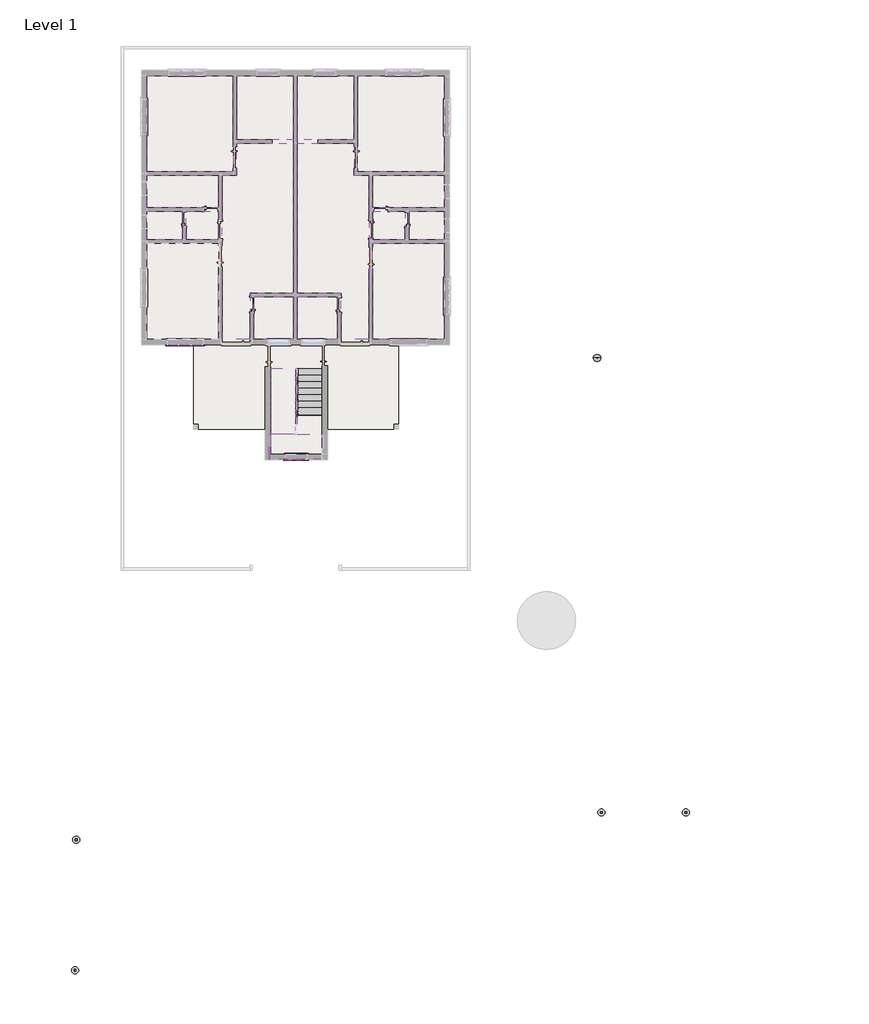
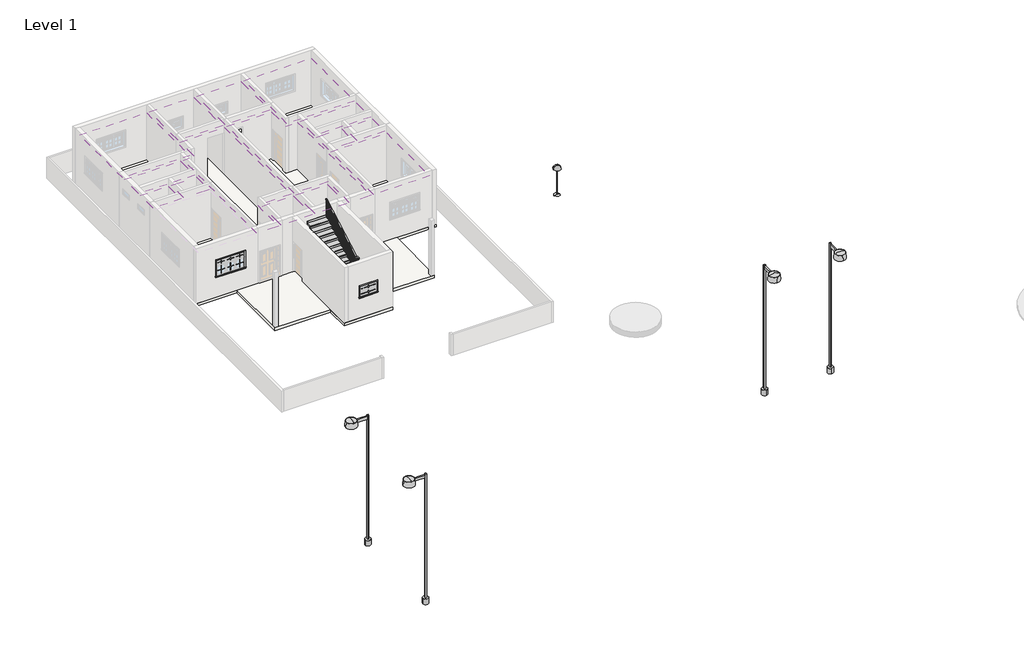
# One storey, part 3 of 4: 15 coverings, 11 proxies, 5 light fixtures, 2 slabs, 2 stair flights, 1 member, 1 railing.
"""IFC4 building model written with IfcOpenShell, lengths in millimetres."""

from ifc_helpers import new_model, si_unit, frame, origin, place, context, project, spatial, polyline, outline, extrude, faceted_brep, transform, mapped, element, save
from components import m_muntin_pattern_2x2_m_muntin_pattern_2x2_be83c6ce, m_muntin_pattern_2x2_m_muntin_pattern_2x2_d2526705, m_muntin_pattern_2x2_m_muntin_pattern_2x2_b257745b, m_muntin_pattern_2x2_m_muntin_pattern_2x2_3c44882e, m_muntin_pattern_2x2_m_muntin_pattern_2x2_c118e93d, m_trim_window_exterior_flat_with_sill_30a8f3cc, m_trim_window_exterior_flat_with_sill_78b3ef69, m_trim_window_interior_flat_picture_frame_87bc748b, m_floor_lamp_hemispheric_100w_277v_4a08ccbb, m_street_light_standard_400w_halogen_120v_204dbcbb, non_monolithic_landing_af9dc4bc, stair_flight_b7621f50, stair_flight_ccf2217f

model = new_model("IFC4")

# Units and contexts
model_context = context("Model", 3, world=origin())
ifc_project = project(units=[si_unit("LENGTHUNIT", "METRE", prefix="MILLI")], contexts=[model_context])

# Site, building, storey
site = spatial("IfcSite", under=ifc_project)
building = spatial("IfcBuilding", under=site)
storey = spatial("IfcBuildingStorey", under=building, Name="Level 1", Elevation=0.0)

# Proxies
placement = place(None, origin())
m_muntin_pattern_2x2_m_muntin_pattern_2x2_shape = m_muntin_pattern_2x2_m_muntin_pattern_2x2_be83c6ce(model_context)
element("IfcBuildingElementProxy", 1, Name="M_Muntin Pattern_2x2 : M_Muntin Pattern_2x2", ObjectType="M_Muntin Pattern_2x2 : M_Muntin Pattern_2x2", at=placement, inside=storey, context=model_context, shape_type="MappedRepresentation", body=[
    mapped(m_muntin_pattern_2x2_m_muntin_pattern_2x2_shape, transform((-11163.0966249, 7920.961641, 1289.05), x_axis=(-1.0, 0.0, 0.0), y_axis=(0.0, -1.0, 0.0), z_axis=(0.0, 0.0, 1.0))),
])
m_muntin_pattern_2x2_m_muntin_pattern_2x2_2_shape = m_muntin_pattern_2x2_m_muntin_pattern_2x2_d2526705(model_context)
element("IfcBuildingElementProxy", 2, Name="M_Muntin Pattern_2x2 : M_Muntin Pattern_2x2", ObjectType="M_Muntin Pattern_2x2 : M_Muntin Pattern_2x2", at=placement, inside=storey, context=model_context, shape_type="MappedRepresentation", body=[
    mapped(m_muntin_pattern_2x2_m_muntin_pattern_2x2_2_shape, transform((-12174.8632915, 7920.961641, 1289.05), x_axis=(1.0, 0.0, 0.0), y_axis=(0.0, 1.0, 0.0), z_axis=(0.0, 0.0, 1.0))),
])
element("IfcBuildingElementProxy", 3, Name="M_Muntin Pattern_2x2 : M_Muntin Pattern_2x2", ObjectType="M_Muntin Pattern_2x2 : M_Muntin Pattern_2x2", at=placement, inside=storey, context=model_context, shape_type="MappedRepresentation", body=[
    mapped(m_muntin_pattern_2x2_m_muntin_pattern_2x2_2_shape, transform((-11668.9799582, 7920.961641, 1289.05), x_axis=(1.0, 0.0, 0.0), y_axis=(0.0, 1.0, 0.0), z_axis=(0.0, 0.0, 1.0))),
])
m_muntin_pattern_2x2_m_muntin_pattern_2x2_3_shape = m_muntin_pattern_2x2_m_muntin_pattern_2x2_b257745b(model_context)
element("IfcBuildingElementProxy", 4, Name="M_Muntin Pattern_2x2 : M_Muntin Pattern_2x2", ObjectType="M_Muntin Pattern_2x2 : M_Muntin Pattern_2x2", at=placement, inside=storey, context=model_context, shape_type="MappedRepresentation", body=[
    mapped(m_muntin_pattern_2x2_m_muntin_pattern_2x2_3_shape, transform((-11668.9799582, 7920.961641, 1889.05), x_axis=(-1.0, 0.0, 0.0), y_axis=(0.0, -1.0, 0.0), z_axis=(0.0, 0.0, 1.0))),
])
element("IfcBuildingElementProxy", 5, Name="M_Muntin Pattern_2x2 : M_Muntin Pattern_2x2", ObjectType="M_Muntin Pattern_2x2 : M_Muntin Pattern_2x2", at=placement, inside=storey, context=model_context, shape_type="MappedRepresentation", body=[
    mapped(m_muntin_pattern_2x2_m_muntin_pattern_2x2_3_shape, transform((-12174.8632915, 7920.961641, 1889.05), x_axis=(-1.0, 0.0, 0.0), y_axis=(0.0, -1.0, 0.0), z_axis=(0.0, 0.0, 1.0))),
])
element("IfcBuildingElementProxy", 6, Name="M_Muntin Pattern_2x2 : M_Muntin Pattern_2x2", ObjectType="M_Muntin Pattern_2x2 : M_Muntin Pattern_2x2", at=placement, inside=storey, context=model_context, shape_type="MappedRepresentation", body=[
    mapped(m_muntin_pattern_2x2_m_muntin_pattern_2x2_3_shape, transform((-11163.0966249, 7920.961641, 1889.05), x_axis=(-1.0, 0.0, 0.0), y_axis=(0.0, -1.0, 0.0), z_axis=(0.0, 0.0, 1.0))),
])
m_muntin_pattern_2x2_m_muntin_pattern_2x2_4_shape = m_muntin_pattern_2x2_m_muntin_pattern_2x2_3c44882e(model_context)
element("IfcBuildingElementProxy", 7, Name="M_Muntin Pattern_2x2 : M_Muntin Pattern_2x2", ObjectType="M_Muntin Pattern_2x2 : M_Muntin Pattern_2x2", at=placement, inside=storey, context=model_context, shape_type="MappedRepresentation", body=[
    mapped(m_muntin_pattern_2x2_m_muntin_pattern_2x2_4_shape, transform((-6927.2581554, 3018.761641, 1589.05), x_axis=(-1.0, 0.0, 0.0), y_axis=(0.0, -1.0, 0.0), z_axis=(0.0, 0.0, 1.0))),
])
m_muntin_pattern_2x2_m_muntin_pattern_2x2_5_shape = m_muntin_pattern_2x2_m_muntin_pattern_2x2_c118e93d(model_context)
element("IfcBuildingElementProxy", 8, Name="M_Muntin Pattern_2x2 : M_Muntin Pattern_2x2", ObjectType="M_Muntin Pattern_2x2 : M_Muntin Pattern_2x2", at=placement, inside=storey, context=model_context, shape_type="MappedRepresentation", body=[
    mapped(m_muntin_pattern_2x2_m_muntin_pattern_2x2_5_shape, transform((-6927.2581554, 3018.761641, 1289.05), x_axis=(-1.0, 0.0, 0.0), y_axis=(0.0, -1.0, 0.0), z_axis=(0.0, 0.0, 1.0))),
])
m_trim_window_exterior_flat_with_sill_shape = m_trim_window_exterior_flat_with_sill_30a8f3cc(model_context)
element("IfcBuildingElementProxy", 9, Name="M_Trim-Window-Exterior-Flat : with Sill", ObjectType="M_Trim-Window-Exterior-Flat : with Sill", at=placement, inside=storey, context=model_context, shape_type="MappedRepresentation", body=[
    mapped(m_trim_window_exterior_flat_with_sill_shape, transform((-11668.9799582, 7911.436641, 2119.2), x_axis=(1.0, 0.0, 0.0), y_axis=(0.0, 0.0, 1.0), z_axis=(0.0, -1.0, 0.0))),
])
m_trim_window_exterior_flat_with_sill_2_shape = m_trim_window_exterior_flat_with_sill_78b3ef69(model_context)
element("IfcBuildingElementProxy", 10, Name="M_Trim-Window-Exterior-Flat : with Sill", ObjectType="M_Trim-Window-Exterior-Flat : with Sill", at=placement, inside=storey, context=model_context, shape_type="MappedRepresentation", body=[
    mapped(m_trim_window_exterior_flat_with_sill_2_shape, transform((-6927.2581554, 3009.236641, 1819.2), x_axis=(1.0, 0.0, 0.0), y_axis=(0.0, 0.0, 1.0), z_axis=(0.0, -1.0, 0.0))),
])
m_trim_window_interior_flat_picture_frame_shape = m_trim_window_interior_flat_picture_frame_87bc748b(model_context)
element("IfcBuildingElementProxy", 11, Name="M_Trim-Window-Interior-Flat : Picture Frame", ObjectType="M_Trim-Window-Interior-Flat : Picture Frame", at=placement, inside=storey, context=model_context, shape_type="MappedRepresentation", body=[
    mapped(m_trim_window_interior_flat_picture_frame_shape, transform((-6927.2581554, 3237.836641, 1819.2), x_axis=(-1.0, 0.0, 0.0), y_axis=(0.0, 0.0, 1.0), z_axis=(0.0, 1.0, 0.0))),
])

# Coverings
element("IfcCovering", 12, ObjectType="2' x 4' ACT System", at=placement, inside=storey, context=model_context, shape_type="SweptSolid", body=[
    extrude(outline(polyline([(-13313.6299582, 19417.636641), (-9630.6299582, 19417.636641), (-9630.6299582, 15302.836641), (-13313.6299582, 15302.836641), (-13313.6299582, 19417.636641)])), frame((0.0, 0.0, 2743.2), z_axis=(0.0, 0.0, 1.0), x_axis=(1.0, 0.0, 0.0)), (0.0, 0.0, 1.0), 57.15),
])
element("IfcCovering", 13, ObjectType="2' x 4' ACT System", at=placement, inside=storey, context=model_context, shape_type="SweptSolid", body=[
    extrude(outline(polyline([(-8894.0299582, 10121.236641), (-8894.0299582, 8140.036641), (-10087.8299582, 8140.036641), (-10087.8299582, 15150.436641), (-9478.2299582, 15150.436641), (-9478.2299582, 16522.036641), (-7039.8299582, 16522.036641), (-7039.8299582, 10121.236641), (-8894.0299582, 10121.236641)])), frame((0.0, 0.0, 2743.2), z_axis=(0.0, 0.0, 1.0), x_axis=(1.0, 0.0, 0.0)), (0.0, 0.0, 1.0), 57.15),
])
element("IfcCovering", 14, ObjectType="2' x 4' ACT System", at=placement, inside=storey, context=model_context, shape_type="SweptSolid", body=[
    extrude(outline(polyline([(-3814.0299582, 8140.036641), (-5007.8299582, 8140.036641), (-5007.8299582, 10121.236641), (-6887.4299582, 10121.236641), (-6887.4299582, 16522.036641), (-4449.0299582, 16522.036641), (-4449.0299582, 15150.436641), (-3814.0299582, 15150.436641), (-3814.0299582, 8140.036641)])), frame((0.0, 0.0, 2743.2), z_axis=(0.0, 0.0, 1.0), x_axis=(1.0, 0.0, 0.0)), (0.0, 0.0, 1.0), 57.15),
])
element("IfcCovering", 15, ObjectType="2' x 4' ACT System", at=placement, inside=storey, context=model_context, shape_type="SweptSolid", body=[
    extrude(outline(polyline([(-6887.4299582, 16674.436641), (-6887.4299582, 19417.636641), (-4449.0299582, 19417.636641), (-4449.0299582, 16674.436641), (-6887.4299582, 16674.436641)])), frame((0.0, 0.0, 2743.2), z_axis=(0.0, 0.0, 1.0), x_axis=(1.0, 0.0, 0.0)), (0.0, 0.0, 1.0), 57.15),
])
element("IfcCovering", 16, ObjectType="2' x 4' ACT System", at=placement, inside=storey, context=model_context, shape_type="SweptSolid", body=[
    extrude(outline(polyline([(-4296.6299582, 15302.836641), (-4296.6299582, 19417.636641), (-588.2299582, 19417.636641), (-588.2299582, 15302.836641), (-4296.6299582, 15302.836641)])), frame((0.0, 0.0, 2743.2), z_axis=(0.0, 0.0, 1.0), x_axis=(1.0, 0.0, 0.0)), (0.0, 0.0, 1.0), 57.15),
])
element("IfcCovering", 17, ObjectType="2' x 4' ACT System", at=placement, inside=storey, context=model_context, shape_type="SweptSolid", body=[
    extrude(outline(polyline([(-588.2299582, 15150.436641), (-588.2299582, 13778.836641), (-3661.6299582, 13778.836641), (-3661.6299582, 15150.436641), (-588.2299582, 15150.436641)])), frame((0.0, 0.0, 2743.2), z_axis=(0.0, 0.0, 1.0), x_axis=(1.0, 0.0, 0.0)), (0.0, 0.0, 1.0), 57.15),
])
element("IfcCovering", 18, ObjectType="2' x 4' ACT System", at=placement, inside=storey, context=model_context, shape_type="SweptSolid", body=[
    extrude(outline(polyline([(-2264.6299582, 12407.236641), (-3661.6299582, 12407.236641), (-3661.6299582, 13626.436641), (-2264.6299582, 13626.436641), (-2264.6299582, 12407.236641)])), frame((0.0, 0.0, 2743.2), z_axis=(0.0, 0.0, 1.0), x_axis=(1.0, 0.0, 0.0)), (0.0, 0.0, 1.0), 57.15),
])
element("IfcCovering", 19, ObjectType="2' x 4' ACT System", at=placement, inside=storey, context=model_context, shape_type="SweptSolid", body=[
    extrude(outline(polyline([(-2112.2299582, 13626.436641), (-588.2299582, 13626.436641), (-588.2299582, 12407.236641), (-2112.2299582, 12407.236641), (-2112.2299582, 13626.436641)])), frame((0.0, 0.0, 2743.2), z_axis=(0.0, 0.0, 1.0), x_axis=(1.0, 0.0, 0.0)), (0.0, 0.0, 1.0), 57.15),
])
element("IfcCovering", 20, ObjectType="2' x 4' ACT System", at=placement, inside=storey, context=model_context, shape_type="SweptSolid", body=[
    extrude(outline(polyline([(-588.2299582, 12254.836641), (-588.2299582, 8140.036641), (-3661.6299582, 8140.036641), (-3661.6299582, 12254.836641), (-588.2299582, 12254.836641)])), frame((0.0, 0.0, 2743.2), z_axis=(0.0, 0.0, 1.0), x_axis=(1.0, 0.0, 0.0)), (0.0, 0.0, 1.0), 57.15),
])
element("IfcCovering", 21, ObjectType="2' x 4' ACT System", at=placement, inside=storey, context=model_context, shape_type="SweptSolid", body=[
    extrude(outline(polyline([(-5160.2299582, 8140.036641), (-6887.4299582, 8140.036641), (-6887.4299582, 9968.836641), (-5160.2299582, 9968.836641), (-5160.2299582, 8140.036641)])), frame((0.0, 0.0, 2743.2), z_axis=(0.0, 0.0, 1.0), x_axis=(1.0, 0.0, 0.0)), (0.0, 0.0, 1.0), 57.15),
])
element("IfcCovering", 22, ObjectType="2' x 4' ACT System", at=placement, inside=storey, context=model_context, shape_type="SweptSolid", body=[
    extrude(outline(polyline([(-7039.8299582, 8140.036641), (-8741.6299582, 8140.036641), (-8741.6299582, 9968.836641), (-7039.8299582, 9968.836641), (-7039.8299582, 8140.036641)])), frame((0.0, 0.0, 2743.2), z_axis=(0.0, 0.0, 1.0), x_axis=(1.0, 0.0, 0.0)), (0.0, 0.0, 1.0), 57.15),
])
element("IfcCovering", 23, ObjectType="2' x 4' ACT System", at=placement, inside=storey, context=model_context, shape_type="SweptSolid", body=[
    extrude(outline(polyline([(-13313.6299582, 12407.236641), (-13313.6299582, 13626.436641), (-11776.9299582, 13626.436641), (-11776.9299582, 12407.236641), (-13313.6299582, 12407.236641)])), frame((0.0, 0.0, 2743.2), z_axis=(0.0, 0.0, 1.0), x_axis=(1.0, 0.0, 0.0)), (0.0, 0.0, 1.0), 57.15),
])
element("IfcCovering", 24, ObjectType="2' x 4' ACT System", at=placement, inside=storey, context=model_context, shape_type="SweptSolid", body=[
    extrude(outline(polyline([(-10240.2299582, 13626.436641), (-10240.2299582, 12407.236641), (-11624.5299582, 12407.236641), (-11624.5299582, 13626.436641), (-10240.2299582, 13626.436641)])), frame((0.0, 0.0, 2743.2), z_axis=(0.0, 0.0, 1.0), x_axis=(1.0, 0.0, 0.0)), (0.0, 0.0, 1.0), 57.15),
])
element("IfcCovering", 25, ObjectType="2' x 4' ACT System", at=placement, inside=storey, context=model_context, shape_type="SweptSolid", body=[
    extrude(outline(polyline([(-10240.2299582, 13778.836641), (-13313.6299582, 13778.836641), (-13313.6299582, 15150.436641), (-10240.2299582, 15150.436641), (-10240.2299582, 13778.836641)])), frame((0.0, 0.0, 2743.2), z_axis=(0.0, 0.0, 1.0), x_axis=(1.0, 0.0, 0.0)), (0.0, 0.0, 1.0), 57.15),
])
element("IfcCovering", 26, ObjectType="2' x 4' ACT System", at=placement, inside=storey, context=model_context, shape_type="SweptSolid", body=[
    extrude(outline(polyline([(-9478.2299582, 16674.436641), (-9478.2299582, 19417.636641), (-7039.8299582, 19417.636641), (-7039.8299582, 16674.436641), (-9478.2299582, 16674.436641)])), frame((0.0, 0.0, 2743.2), z_axis=(0.0, 0.0, 1.0), x_axis=(1.0, 0.0, 0.0)), (0.0, 0.0, 1.0), 57.15),
])

# Light fixtures
m_floor_lamp_hemispheric_100w_277v_shape = m_floor_lamp_hemispheric_100w_277v_4a08ccbb(model_context)
element("IfcLightFixture", 27, ObjectType="M_Floor Lamp - Hemispheric : 100W - 277V", at=placement, inside=storey, context=model_context, shape_type="MappedRepresentation", body=[
    mapped(m_floor_lamp_hemispheric_100w_277v_shape, transform((5939.5700418, 7352.636641, -141.6133158), x_axis=(1.0, 0.0, 0.0), y_axis=(0.0, 1.0, 0.0), z_axis=(0.0, 0.0, 1.0))),
])
m_street_light_standard_400w_halogen_120v_shape = m_street_light_standard_400w_halogen_120v_204dbcbb(model_context)
element("IfcLightFixture", 28, ObjectType="M_Street Light - Standard : 400W Halogen - 120V", at=placement, inside=storey, context=model_context, shape_type="MappedRepresentation", body=[
    mapped(m_street_light_standard_400w_halogen_120v_shape, transform((6127.5437539, -12075.4373856, 0.0), x_axis=(0.0, 1.0, 0.0), y_axis=(-1.0, 0.0, 0.0), z_axis=(0.0, 0.0, 1.0))),
])
element("IfcLightFixture", 29, ObjectType="M_Street Light - Standard : 400W Halogen - 120V", at=placement, inside=storey, context=model_context, shape_type="MappedRepresentation", body=[
    mapped(m_street_light_standard_400w_halogen_120v_shape, transform((9737.5760678, -12075.4373856, 0.0), x_axis=(0.0, 1.0, 0.0), y_axis=(-1.0, 0.0, 0.0), z_axis=(0.0, 0.0, 1.0))),
])
element("IfcLightFixture", 30, ObjectType="M_Street Light - Standard : 400W Halogen - 480V", at=placement, inside=storey, context=model_context, shape_type="MappedRepresentation", body=[
    mapped(m_street_light_standard_400w_halogen_120v_shape, transform((-16336.2299582, -13246.763359, -152.4), x_axis=(1.0, 0.0, 0.0), y_axis=(0.0, 1.0, 0.0), z_axis=(0.0, 0.0, 1.0))),
])
element("IfcLightFixture", 31, ObjectType="M_Street Light - Standard : 400W Halogen - 480V", at=placement, inside=storey, context=model_context, shape_type="MappedRepresentation", body=[
    mapped(m_street_light_standard_400w_halogen_120v_shape, transform((-16386.7490049, -18825.9765537, -152.4), x_axis=(1.0, 0.0, 0.0), y_axis=(0.0, 1.0, 0.0), z_axis=(0.0, 0.0, 1.0))),
])

# Member
element("IfcMember", 32, ObjectType="Stringer - 2\" Width", at=placement, inside=storey, context=model_context, shape_type="SweptSolid", body=[
    extrude(outline(polyline([(-8082.9581554, 4095.086641), (-8032.1581554, 4095.086641), (-8032.1581554, 3028.286641), (-8082.9581554, 3028.286641), (-8082.9581554, 4095.086641)])), frame((0.0, 0.0, 1524.0), z_axis=(0.0, 0.0, 1.0), x_axis=(1.0, 0.0, 0.0)), (0.0, 0.0, 1.0), 304.8),
])

# Railing
element("IfcRailing", 33, ObjectType="Handrail - Rectangular", at=placement, inside=storey, context=model_context, shape_type="SolidModel", body=[
    faceted_brep([(-6838.3581554, 6889.086641, 1073.7272727), (-6838.3581554, 6889.086641, 1015.2480499), (-6889.1581554, 6889.086641, 1015.2480499), (-6889.1581554, 6889.086641, 1073.7272727), (-6838.3581554, 4171.286641, 2623.5471074), (-6838.3581554, 4120.486641, 2594.0364797), (-6889.1581554, 4120.486641, 2594.0364797), (-6889.1581554, 4171.286641, 2623.5471074), (-6838.3581554, 4171.286641, 2667.0), (-6838.3581554, 4120.486641, 2616.2), (-6889.1581554, 4120.486641, 2616.2), (-6889.1581554, 4171.286641, 2667.0), (-6838.3581554, 4044.286641, 2667.0), (-6838.3581554, 4044.286641, 2616.2), (-6889.1581554, 4095.086641, 2616.2), (-6889.1581554, 4095.086641, 2667.0), (-6965.3581554, 4044.286641, 2667.0), (-6965.3581554, 4044.286641, 2616.2), (-6965.3581554, 4095.086641, 2616.2), (-6965.3581554, 4095.086641, 2667.0), (-6990.7581554, 4044.286641, 2667.0), (-6990.7581554, 4095.086641, 2667.0), (-6990.7581554, 4095.086641, 2616.2), (-6990.7581554, 4044.286641, 2616.2)], [[[0, 1, 2, 3]], [[1, 0, 4, 5]], [[2, 1, 5, 6]], [[3, 2, 6, 7]], [[0, 3, 7, 4]], [[5, 4, 8, 9]], [[6, 5, 9, 10]], [[7, 6, 10, 11]], [[4, 7, 11, 8]], [[9, 8, 12, 13]], [[10, 9, 13, 14]], [[11, 10, 14, 15]], [[8, 11, 15, 12]], [[13, 12, 16, 17]], [[14, 13, 17, 18]], [[15, 14, 18, 19]], [[12, 15, 19, 16]], [[20, 21, 22, 23]], [[17, 16, 20, 23]], [[18, 17, 23, 22]], [[19, 18, 22, 21]], [[16, 19, 21, 20]]]),
    faceted_brep([(-6965.3581554, 4044.286641, 2667.0), (-7016.1581554, 4044.286641, 2616.2), (-7016.1581554, 4095.086641, 2616.2), (-6965.3581554, 4095.086641, 2667.0), (-6965.3581554, 4044.286641, 2797.3586777), (-6965.3581554, 4095.086641, 2767.8480499), (-7016.1581554, 4095.086641, 2767.8480499), (-7016.1581554, 4044.286641, 2797.3586777)], [[[0, 1, 2, 3]], [[4, 5, 6, 7]], [[1, 0, 4, 7]], [[2, 1, 7, 6]], [[3, 2, 6, 5]], [[0, 3, 5, 4]]]),
    faceted_brep([(-7016.1581554, 4044.286641, 2797.3586777), (-7016.1581554, 4095.086641, 2767.8480499), (-6965.3581554, 4095.086641, 2767.8480499), (-6965.3581554, 4044.286641, 2797.3586777), (-7016.1581554, 6889.086641, 4419.6), (-6965.3581554, 6889.086641, 4419.6), (-6965.3581554, 6889.086641, 4361.1207772), (-7016.1581554, 6889.086641, 4361.1207772)], [[[0, 1, 2, 3]], [[4, 5, 6, 7]], [[1, 0, 4, 7]], [[2, 1, 7, 6]], [[3, 2, 6, 5]], [[0, 3, 5, 4]]]),
    extrude(outline(polyline([(6803.361641, 4312.2362731), (6822.411641, 4323.0994962), (6822.411641, 3345.8727273), (6803.361641, 3345.8727273), (6803.361641, 4312.2362731)])), frame((-7000.2831554, 0.0, 0.0), z_axis=(1.0, 0.0, 0.0), x_axis=(0.0, 1.0, 0.0)), (0.0, 0.0, 1.0), 19.05),
    extrude(outline(polyline([(6701.761641, 4254.299083), (6720.811641, 4265.1623061), (6720.811641, 3345.8727273), (6701.761641, 3345.8727273), (6701.761641, 4254.299083)])), frame((-7000.2831554, 0.0, 0.0), z_axis=(1.0, 0.0, 0.0), x_axis=(0.0, 1.0, 0.0)), (0.0, 0.0, 1.0), 19.05),
    extrude(outline(polyline([(6600.161641, 4196.3618929), (6619.211641, 4207.225116), (6619.211641, 3345.8727273), (6600.161641, 3345.8727273), (6600.161641, 4196.3618929)])), frame((-7000.2831554, 0.0, 0.0), z_axis=(1.0, 0.0, 0.0), x_axis=(0.0, 1.0, 0.0)), (0.0, 0.0, 1.0), 19.05),
    extrude(outline(polyline([(6498.561641, 4138.4247028), (6517.611641, 4149.287926), (6517.611641, 3186.5454545), (6498.561641, 3186.5454545), (6498.561641, 4138.4247028)])), frame((-7000.2831554, 0.0, 0.0), z_axis=(1.0, 0.0, 0.0), x_axis=(0.0, 1.0, 0.0)), (0.0, 0.0, 1.0), 19.05),
    extrude(outline(polyline([(6396.961641, 4080.4875127), (6416.011641, 4091.3507359), (6416.011641, 3186.5454545), (6396.961641, 3186.5454545), (6396.961641, 4080.4875127)])), frame((-7000.2831554, 0.0, 0.0), z_axis=(1.0, 0.0, 0.0), x_axis=(0.0, 1.0, 0.0)), (0.0, 0.0, 1.0), 19.05),
    extrude(outline(polyline([(6295.361641, 4022.5503227), (6314.411641, 4033.4135458), (6314.411641, 3027.2181818), (6295.361641, 3027.2181818), (6295.361641, 4022.5503227)])), frame((-7000.2831554, 0.0, 0.0), z_axis=(1.0, 0.0, 0.0), x_axis=(0.0, 1.0, 0.0)), (0.0, 0.0, 1.0), 19.05),
    extrude(outline(polyline([(6193.761641, 3964.6131326), (6212.811641, 3975.4763557), (6212.811641, 3027.2181818), (6193.761641, 3027.2181818), (6193.761641, 3964.6131326)])), frame((-7000.2831554, 0.0, 0.0), z_axis=(1.0, 0.0, 0.0), x_axis=(0.0, 1.0, 0.0)), (0.0, 0.0, 1.0), 19.05),
    extrude(outline(polyline([(6092.161641, 3906.6759425), (6111.211641, 3917.5391656), (6111.211641, 3027.2181818), (6092.161641, 3027.2181818), (6092.161641, 3906.6759425)])), frame((-7000.2831554, 0.0, 0.0), z_axis=(1.0, 0.0, 0.0), x_axis=(0.0, 1.0, 0.0)), (0.0, 0.0, 1.0), 19.05),
    extrude(outline(polyline([(5990.561641, 3848.7387524), (6009.611641, 3859.6019756), (6009.611641, 2867.8909091), (5990.561641, 2867.8909091), (5990.561641, 3848.7387524)])), frame((-7000.2831554, 0.0, 0.0), z_axis=(1.0, 0.0, 0.0), x_axis=(0.0, 1.0, 0.0)), (0.0, 0.0, 1.0), 19.05),
    extrude(outline(polyline([(5888.961641, 3790.8015623), (5908.011641, 3801.6647855), (5908.011641, 2867.8909091), (5888.961641, 2867.8909091), (5888.961641, 3790.8015623)])), frame((-7000.2831554, 0.0, 0.0), z_axis=(1.0, 0.0, 0.0), x_axis=(0.0, 1.0, 0.0)), (0.0, 0.0, 1.0), 19.05),
    extrude(outline(polyline([(5787.361641, 3732.8643722), (5806.411641, 3743.7275954), (5806.411641, 2867.8909091), (5787.361641, 2867.8909091), (5787.361641, 3732.8643722)])), frame((-7000.2831554, 0.0, 0.0), z_axis=(1.0, 0.0, 0.0), x_axis=(0.0, 1.0, 0.0)), (0.0, 0.0, 1.0), 19.05),
    extrude(outline(polyline([(5685.761641, 3674.9271822), (5704.811641, 3685.7904053), (5704.811641, 2708.5636364), (5685.761641, 2708.5636364), (5685.761641, 3674.9271822)])), frame((-7000.2831554, 0.0, 0.0), z_axis=(1.0, 0.0, 0.0), x_axis=(0.0, 1.0, 0.0)), (0.0, 0.0, 1.0), 19.05),
    extrude(outline(polyline([(5584.161641, 3616.9899921), (5603.211641, 3627.8532152), (5603.211641, 2708.5636364), (5584.161641, 2708.5636364), (5584.161641, 3616.9899921)])), frame((-7000.2831554, 0.0, 0.0), z_axis=(1.0, 0.0, 0.0), x_axis=(0.0, 1.0, 0.0)), (0.0, 0.0, 1.0), 19.05),
    extrude(outline(polyline([(5482.561641, 3559.052802), (5501.611641, 3569.9160251), (5501.611641, 2708.5636364), (5482.561641, 2708.5636364), (5482.561641, 3559.052802)])), frame((-7000.2831554, 0.0, 0.0), z_axis=(1.0, 0.0, 0.0), x_axis=(0.0, 1.0, 0.0)), (0.0, 0.0, 1.0), 19.05),
    extrude(outline(polyline([(5380.961641, 3501.1156119), (5400.011641, 3511.9788351), (5400.011641, 2549.2363636), (5380.961641, 2549.2363636), (5380.961641, 3501.1156119)])), frame((-7000.2831554, 0.0, 0.0), z_axis=(1.0, 0.0, 0.0), x_axis=(0.0, 1.0, 0.0)), (0.0, 0.0, 1.0), 19.05),
    extrude(outline(polyline([(5279.361641, 3443.1784218), (5298.411641, 3454.041645), (5298.411641, 2549.2363636), (5279.361641, 2549.2363636), (5279.361641, 3443.1784218)])), frame((-7000.2831554, 0.0, 0.0), z_axis=(1.0, 0.0, 0.0), x_axis=(0.0, 1.0, 0.0)), (0.0, 0.0, 1.0), 19.05),
    extrude(outline(polyline([(5177.761641, 3385.2412318), (5196.811641, 3396.1044549), (5196.811641, 2389.9090909), (5177.761641, 2389.9090909), (5177.761641, 3385.2412318)])), frame((-7000.2831554, 0.0, 0.0), z_axis=(1.0, 0.0, 0.0), x_axis=(0.0, 1.0, 0.0)), (0.0, 0.0, 1.0), 19.05),
    extrude(outline(polyline([(5076.161641, 3327.3040417), (5095.211641, 3338.1672648), (5095.211641, 2389.9090909), (5076.161641, 2389.9090909), (5076.161641, 3327.3040417)])), frame((-7000.2831554, 0.0, 0.0), z_axis=(1.0, 0.0, 0.0), x_axis=(0.0, 1.0, 0.0)), (0.0, 0.0, 1.0), 19.05),
    extrude(outline(polyline([(4974.561641, 3269.3668516), (4993.611641, 3280.2300747), (4993.611641, 2389.9090909), (4974.561641, 2389.9090909), (4974.561641, 3269.3668516)])), frame((-7000.2831554, 0.0, 0.0), z_axis=(1.0, 0.0, 0.0), x_axis=(0.0, 1.0, 0.0)), (0.0, 0.0, 1.0), 19.05),
    extrude(outline(polyline([(4872.961641, 3211.4296615), (4892.011641, 3222.2928846), (4892.011641, 2230.5818182), (4872.961641, 2230.5818182), (4872.961641, 3211.4296615)])), frame((-7000.2831554, 0.0, 0.0), z_axis=(1.0, 0.0, 0.0), x_axis=(0.0, 1.0, 0.0)), (0.0, 0.0, 1.0), 19.05),
    extrude(outline(polyline([(4771.361641, 3153.4924714), (4790.411641, 3164.3556946), (4790.411641, 2230.5818182), (4771.361641, 2230.5818182), (4771.361641, 3153.4924714)])), frame((-7000.2831554, 0.0, 0.0), z_axis=(1.0, 0.0, 0.0), x_axis=(0.0, 1.0, 0.0)), (0.0, 0.0, 1.0), 19.05),
    extrude(outline(polyline([(4669.761641, 3095.5552813), (4688.811641, 3106.4185045), (4688.811641, 2230.5818182), (4669.761641, 2230.5818182), (4669.761641, 3095.5552813)])), frame((-7000.2831554, 0.0, 0.0), z_axis=(1.0, 0.0, 0.0), x_axis=(0.0, 1.0, 0.0)), (0.0, 0.0, 1.0), 19.05),
    extrude(outline(polyline([(4568.161641, 3037.6180913), (4587.211641, 3048.4813144), (4587.211641, 2071.2545455), (4568.161641, 2071.2545455), (4568.161641, 3037.6180913)])), frame((-7000.2831554, 0.0, 0.0), z_axis=(1.0, 0.0, 0.0), x_axis=(0.0, 1.0, 0.0)), (0.0, 0.0, 1.0), 19.05),
    extrude(outline(polyline([(4466.561641, 2979.6809012), (4485.611641, 2990.5441243), (4485.611641, 2071.2545455), (4466.561641, 2071.2545455), (4466.561641, 2979.6809012)])), frame((-7000.2831554, 0.0, 0.0), z_axis=(1.0, 0.0, 0.0), x_axis=(0.0, 1.0, 0.0)), (0.0, 0.0, 1.0), 19.05),
    extrude(outline(polyline([(4364.961641, 2921.7437111), (4384.011641, 2932.6069342), (4384.011641, 2071.2545455), (4364.961641, 2071.2545455), (4364.961641, 2921.7437111)])), frame((-7000.2831554, 0.0, 0.0), z_axis=(1.0, 0.0, 0.0), x_axis=(0.0, 1.0, 0.0)), (0.0, 0.0, 1.0), 19.05),
    extrude(outline(polyline([(4263.361641, 2863.806521), (4282.411641, 2874.6697441), (4282.411641, 1911.9272727), (4263.361641, 1911.9272727), (4263.361641, 2863.806521)])), frame((-7000.2831554, 0.0, 0.0), z_axis=(1.0, 0.0, 0.0), x_axis=(0.0, 1.0, 0.0)), (0.0, 0.0, 1.0), 19.05),
    extrude(outline(polyline([(4161.761641, 2805.8693309), (4180.811641, 2816.7325541), (4180.811641, 1911.9272727), (4161.761641, 1911.9272727), (4161.761641, 2805.8693309)])), frame((-7000.2831554, 0.0, 0.0), z_axis=(1.0, 0.0, 0.0), x_axis=(0.0, 1.0, 0.0)), (0.0, 0.0, 1.0), 19.05),
    extrude(outline(polyline([(-6955.8331554, 4079.211641), (-6955.8331554, 4060.161641), (-6974.8831554, 4060.161641), (-6974.8831554, 4079.211641), (-6955.8331554, 4079.211641)])), frame((0.0, 0.0, 1752.6), z_axis=(0.0, 0.0, 1.0), x_axis=(1.0, 0.0, 0.0)), (0.0, 0.0, 1.0), 863.6),
    extrude(outline(polyline([(-6873.2831554, 4155.411641), (-6854.2331554, 4155.411641), (-6854.2331554, 4136.361641), (-6873.2831554, 4136.361641), (-6873.2831554, 4155.411641)])), frame((0.0, 0.0, 1593.2727273), z_axis=(0.0, 0.0, 1.0), x_axis=(1.0, 0.0, 0.0)), (0.0, 0.0, 1.0), 1022.9272727),
    extrude(outline(polyline([(4237.961641, 2527.0466037), (4257.011641, 2516.1833805), (4257.011641, 1593.2727273), (4237.961641, 1593.2727273), (4237.961641, 2527.0466037)])), frame((-6873.2831554, 0.0, 0.0), z_axis=(1.0, 0.0, 0.0), x_axis=(0.0, 1.0, 0.0)), (0.0, 0.0, 1.0), 19.05),
    extrude(outline(polyline([(4339.561641, 2469.1094136), (4358.611641, 2458.2461904), (4358.611641, 1593.2727273), (4339.561641, 1593.2727273), (4339.561641, 2469.1094136)])), frame((-6873.2831554, 0.0, 0.0), z_axis=(1.0, 0.0, 0.0), x_axis=(0.0, 1.0, 0.0)), (0.0, 0.0, 1.0), 19.05),
    extrude(outline(polyline([(4441.161641, 2411.1722235), (4460.211641, 2400.3090003), (4460.211641, 1433.9454545), (4441.161641, 1433.9454545), (4441.161641, 2411.1722235)])), frame((-6873.2831554, 0.0, 0.0), z_axis=(1.0, 0.0, 0.0), x_axis=(0.0, 1.0, 0.0)), (0.0, 0.0, 1.0), 19.05),
    extrude(outline(polyline([(4542.761641, 2353.2350334), (4561.811641, 2342.3718103), (4561.811641, 1433.9454545), (4542.761641, 1433.9454545), (4542.761641, 2353.2350334)])), frame((-6873.2831554, 0.0, 0.0), z_axis=(1.0, 0.0, 0.0), x_axis=(0.0, 1.0, 0.0)), (0.0, 0.0, 1.0), 19.05),
    extrude(outline(polyline([(4644.361641, 2295.2978433), (4663.411641, 2284.4346202), (4663.411641, 1433.9454545), (4644.361641, 1433.9454545), (4644.361641, 2295.2978433)])), frame((-6873.2831554, 0.0, 0.0), z_axis=(1.0, 0.0, 0.0), x_axis=(0.0, 1.0, 0.0)), (0.0, 0.0, 1.0), 19.05),
    extrude(outline(polyline([(4745.961641, 2237.3606532), (4765.011641, 2226.4974301), (4765.011641, 1274.6181818), (4745.961641, 1274.6181818), (4745.961641, 2237.3606532)])), frame((-6873.2831554, 0.0, 0.0), z_axis=(1.0, 0.0, 0.0), x_axis=(0.0, 1.0, 0.0)), (0.0, 0.0, 1.0), 19.05),
    extrude(outline(polyline([(4847.561641, 2179.4234632), (4866.611641, 2168.56024), (4866.611641, 1274.6181818), (4847.561641, 1274.6181818), (4847.561641, 2179.4234632)])), frame((-6873.2831554, 0.0, 0.0), z_axis=(1.0, 0.0, 0.0), x_axis=(0.0, 1.0, 0.0)), (0.0, 0.0, 1.0), 19.05),
    extrude(outline(polyline([(4949.161641, 2121.4862731), (4968.211641, 2110.6230499), (4968.211641, 1115.2909091), (4949.161641, 1115.2909091), (4949.161641, 2121.4862731)])), frame((-6873.2831554, 0.0, 0.0), z_axis=(1.0, 0.0, 0.0), x_axis=(0.0, 1.0, 0.0)), (0.0, 0.0, 1.0), 19.05),
    extrude(outline(polyline([(5050.761641, 2063.549083), (5069.811641, 2052.6858598), (5069.811641, 1115.2909091), (5050.761641, 1115.2909091), (5050.761641, 2063.549083)])), frame((-6873.2831554, 0.0, 0.0), z_axis=(1.0, 0.0, 0.0), x_axis=(0.0, 1.0, 0.0)), (0.0, 0.0, 1.0), 19.05),
    extrude(outline(polyline([(5152.361641, 2005.6118929), (5171.411641, 1994.7486698), (5171.411641, 1115.2909091), (5152.361641, 1115.2909091), (5152.361641, 2005.6118929)])), frame((-6873.2831554, 0.0, 0.0), z_axis=(1.0, 0.0, 0.0), x_axis=(0.0, 1.0, 0.0)), (0.0, 0.0, 1.0), 19.05),
    extrude(outline(polyline([(5253.961641, 1947.6747028), (5273.011641, 1936.8114797), (5273.011641, 955.9636364), (5253.961641, 955.9636364), (5253.961641, 1947.6747028)])), frame((-6873.2831554, 0.0, 0.0), z_axis=(1.0, 0.0, 0.0), x_axis=(0.0, 1.0, 0.0)), (0.0, 0.0, 1.0), 19.05),
    extrude(outline(polyline([(5355.561641, 1889.7375127), (5374.611641, 1878.8742896), (5374.611641, 955.9636364), (5355.561641, 955.9636364), (5355.561641, 1889.7375127)])), frame((-6873.2831554, 0.0, 0.0), z_axis=(1.0, 0.0, 0.0), x_axis=(0.0, 1.0, 0.0)), (0.0, 0.0, 1.0), 19.05),
    extrude(outline(polyline([(5457.161641, 1831.8003227), (5476.211641, 1820.9370995), (5476.211641, 955.9636364), (5457.161641, 955.9636364), (5457.161641, 1831.8003227)])), frame((-6873.2831554, 0.0, 0.0), z_axis=(1.0, 0.0, 0.0), x_axis=(0.0, 1.0, 0.0)), (0.0, 0.0, 1.0), 19.05),
    extrude(outline(polyline([(5558.761641, 1773.8631326), (5577.811641, 1762.9999094), (5577.811641, 796.6363636), (5558.761641, 796.6363636), (5558.761641, 1773.8631326)])), frame((-6873.2831554, 0.0, 0.0), z_axis=(1.0, 0.0, 0.0), x_axis=(0.0, 1.0, 0.0)), (0.0, 0.0, 1.0), 19.05),
    extrude(outline(polyline([(5660.361641, 1715.9259425), (5679.411641, 1705.0627194), (5679.411641, 796.6363636), (5660.361641, 796.6363636), (5660.361641, 1715.9259425)])), frame((-6873.2831554, 0.0, 0.0), z_axis=(1.0, 0.0, 0.0), x_axis=(0.0, 1.0, 0.0)), (0.0, 0.0, 1.0), 19.05),
    extrude(outline(polyline([(5761.961641, 1657.9887524), (5781.011641, 1647.1255293), (5781.011641, 796.6363636), (5761.961641, 796.6363636), (5761.961641, 1657.9887524)])), frame((-6873.2831554, 0.0, 0.0), z_axis=(1.0, 0.0, 0.0), x_axis=(0.0, 1.0, 0.0)), (0.0, 0.0, 1.0), 19.05),
    extrude(outline(polyline([(5863.561641, 1600.0515623), (5882.611641, 1589.1883392), (5882.611641, 637.3090909), (5863.561641, 637.3090909), (5863.561641, 1600.0515623)])), frame((-6873.2831554, 0.0, 0.0), z_axis=(1.0, 0.0, 0.0), x_axis=(0.0, 1.0, 0.0)), (0.0, 0.0, 1.0), 19.05),
    extrude(outline(polyline([(5965.161641, 1542.1143722), (5984.211641, 1531.2511491), (5984.211641, 637.3090909), (5965.161641, 637.3090909), (5965.161641, 1542.1143722)])), frame((-6873.2831554, 0.0, 0.0), z_axis=(1.0, 0.0, 0.0), x_axis=(0.0, 1.0, 0.0)), (0.0, 0.0, 1.0), 19.05),
    extrude(outline(polyline([(6066.761641, 1484.1771822), (6085.811641, 1473.313959), (6085.811641, 477.9818182), (6066.761641, 477.9818182), (6066.761641, 1484.1771822)])), frame((-6873.2831554, 0.0, 0.0), z_axis=(1.0, 0.0, 0.0), x_axis=(0.0, 1.0, 0.0)), (0.0, 0.0, 1.0), 19.05),
    extrude(outline(polyline([(6168.361641, 1426.2399921), (6187.411641, 1415.3767689), (6187.411641, 477.9818182), (6168.361641, 477.9818182), (6168.361641, 1426.2399921)])), frame((-6873.2831554, 0.0, 0.0), z_axis=(1.0, 0.0, 0.0), x_axis=(0.0, 1.0, 0.0)), (0.0, 0.0, 1.0), 19.05),
    extrude(outline(polyline([(6269.961641, 1368.302802), (6289.011641, 1357.4395789), (6289.011641, 477.9818182), (6269.961641, 477.9818182), (6269.961641, 1368.302802)])), frame((-6873.2831554, 0.0, 0.0), z_axis=(1.0, 0.0, 0.0), x_axis=(0.0, 1.0, 0.0)), (0.0, 0.0, 1.0), 19.05),
    extrude(outline(polyline([(6371.561641, 1310.3656119), (6390.611641, 1299.5023888), (6390.611641, 318.6545455), (6371.561641, 318.6545455), (6371.561641, 1310.3656119)])), frame((-6873.2831554, 0.0, 0.0), z_axis=(1.0, 0.0, 0.0), x_axis=(0.0, 1.0, 0.0)), (0.0, 0.0, 1.0), 19.05),
    extrude(outline(polyline([(6473.161641, 1252.4284218), (6492.211641, 1241.5651987), (6492.211641, 318.6545455), (6473.161641, 318.6545455), (6473.161641, 1252.4284218)])), frame((-6873.2831554, 0.0, 0.0), z_axis=(1.0, 0.0, 0.0), x_axis=(0.0, 1.0, 0.0)), (0.0, 0.0, 1.0), 19.05),
    extrude(outline(polyline([(6574.761641, 1194.4912318), (6593.811641, 1183.6280086), (6593.811641, 318.6545455), (6574.761641, 318.6545455), (6574.761641, 1194.4912318)])), frame((-6873.2831554, 0.0, 0.0), z_axis=(1.0, 0.0, 0.0), x_axis=(0.0, 1.0, 0.0)), (0.0, 0.0, 1.0), 19.05),
    extrude(outline(polyline([(6676.361641, 1136.5540417), (6695.411641, 1125.6908185), (6695.411641, 159.3272727), (6676.361641, 159.3272727), (6676.361641, 1136.5540417)])), frame((-6873.2831554, 0.0, 0.0), z_axis=(1.0, 0.0, 0.0), x_axis=(0.0, 1.0, 0.0)), (0.0, 0.0, 1.0), 19.05),
    extrude(outline(polyline([(6777.961641, 1078.6168516), (6797.011641, 1067.7536284), (6797.011641, 159.3272727), (6777.961641, 159.3272727), (6777.961641, 1078.6168516)])), frame((-6873.2831554, 0.0, 0.0), z_axis=(1.0, 0.0, 0.0), x_axis=(0.0, 1.0, 0.0)), (0.0, 0.0, 1.0), 19.05),
    extrude(outline(polyline([(-6981.2331554, 4079.211641), (-6981.2331554, 4060.161641), (-7000.2831554, 4060.161641), (-7000.2831554, 4079.211641), (-6981.2331554, 4079.211641)])), frame((0.0, 0.0, 1752.6), z_axis=(0.0, 0.0, 1.0), x_axis=(1.0, 0.0, 0.0)), (0.0, 0.0, 1.0), 863.6),
    extrude(outline(polyline([(-6873.2831554, 4079.211641), (-6854.2331554, 4079.211641), (-6854.2331554, 4060.161641), (-6873.2831554, 4060.161641), (-6873.2831554, 4079.211641)])), frame((0.0, 0.0, 1752.6), z_axis=(0.0, 0.0, 1.0), x_axis=(1.0, 0.0, 0.0)), (0.0, 0.0, 1.0), 863.6),
    extrude(outline(polyline([(6870.036641, 4350.2575541), (6889.086641, 4361.1207772), (6889.086641, 3345.8727273), (6870.036641, 3345.8727273), (6870.036641, 4350.2575541)])), frame((-7000.2831554, 0.0, 0.0), z_axis=(1.0, 0.0, 0.0), x_axis=(0.0, 1.0, 0.0)), (0.0, 0.0, 1.0), 19.05),
    extrude(outline(polyline([(6803.361641, 1064.1325541), (6822.411641, 1053.2693309), (6822.411641, 159.3272727), (6803.361641, 159.3272727), (6803.361641, 1064.1325541)])), frame((-6873.2831554, 0.0, 0.0), z_axis=(1.0, 0.0, 0.0), x_axis=(0.0, 1.0, 0.0)), (0.0, 0.0, 1.0), 19.05),
])

# Slabs
element("IfcSlab", 34, ObjectType="Generic - 6\"", at=placement, inside=storey, context=model_context, shape_type="SweptSolid", body=[
    extrude(outline(polyline([(-13542.2299582, 7911.436641), (-13542.2299582, 19646.236641), (-359.6299582, 19646.236641), (-359.6299582, 7911.436641), (-2545.7581554, 7911.436641), (-2545.7581554, 4304.636641), (-5593.7581554, 4304.636641), (-5593.7581554, 3009.236641), (-8260.7581554, 3009.236641), (-8260.7581554, 4304.636641), (-11308.7581554, 4304.636641), (-11308.7581554, 7911.436641), (-13542.2299582, 7911.436641)])), frame((0.0, 0.0, -152.4), z_axis=(0.0, 0.0, 1.0), x_axis=(1.0, 0.0, 0.0)), (0.0, 0.0, 1.0), 152.4),
])
non_monolithic_landing_shape = non_monolithic_landing_af9dc4bc(model_context)
element("IfcSlab", 35, ObjectType="Non-Monolithic Landing", at=placement, inside=storey, context=model_context, shape_type="MappedRepresentation", body=[
    mapped(non_monolithic_landing_shape, transform((0.0, 0.0, 0.0), x_axis=(1.0, 0.0, 0.0), y_axis=(0.0, 1.0, 0.0), z_axis=(0.0, 0.0, 1.0))),
])

# Stair flights
stair_flight_shape = stair_flight_b7621f50(model_context)
element("IfcStairFlight", 36, ObjectType="2\" Tread 1\" Nosing 1/4\" Riser", at=placement, inside=storey, context=model_context, shape_type="MappedRepresentation", body=[
    mapped(stair_flight_shape, transform((0.0, 0.0, 0.0), x_axis=(1.0, 0.0, 0.0), y_axis=(0.0, 1.0, 0.0), z_axis=(0.0, 0.0, 1.0))),
])
stair_flight_2_shape = stair_flight_ccf2217f(model_context)
element("IfcStairFlight", 37, ObjectType="2\" Tread 1\" Nosing 1/4\" Riser", at=placement, inside=storey, context=model_context, shape_type="MappedRepresentation", body=[
    mapped(stair_flight_2_shape, transform((0.0, 0.0, 0.0), x_axis=(1.0, 0.0, 0.0), y_axis=(0.0, 1.0, 0.0), z_axis=(0.0, 0.0, 1.0))),
])

save(model, "model.ifc")

# Revit data of these elements
# Type "M_Muntin Pattern_2x2 : M_Muntin Pattern_2x2"
#   Width [instance default] = 3' - 11.24409"
#   Thickness = 0' - 0 1/2"
#   Height [instance default] = 3' - 11.24409"
#   Distance = 0' - 0 3/4"
#   Interior Material [instance default] = none
#   Exterior Material [instance default] = none
#   Default Elevation = 0
# Type "M_Trim-Window-Exterior-Flat : with Sill"
#   Trim Width = 0' - 2.3622"
#   Trim Thickness_Picture Frame = 0' - 1.1811"
#   Trim Thickness_with Sill = 0' - 0 3/4"
#   Sill Thickness = 0' - 1.1811"
#   Opening Width [instance default] = 1' - 11.62205"
#   Opening Height [instance default] = 2' - 11.43307"
#   Default Elevation = 3' - 11.24409"
#   Sill = yes
#   Picture Frame = no
#   Trim Material [instance default] = none
# Type "M_Trim-Window-Interior-Flat : Picture Frame"
#   Trim Thickness_Picture Frame = 0' - 1.1811"
#   Trim Width = 0' - 2.3622"
#   Trim Thickness_with Sill = 0' - 0.7874"
#   Sill Thickness = 0' - 1.1811"
#   Opening Width [instance default] = 1' - 11.62205"
#   Opening Height [instance default] = 2' - 11.43307"
#   Default Elevation = 3' - 11.24409"
#   Sill = no
#   Picture Frame = yes
#   Trim Material [instance default] = none
# Type "2' x 4' ACT System"
#   Assembly Code = "C3030210"
#   built-in parameter 1002203 = 1 (stored number, unit not read)
#   built-in parameter 1002202 = 1 (stored number, unit not read)
#   Layers, outside or top first: 0' - 1 5/8" "Default" (function 1); 0' - 0 5/8" "Acoustic Ceiling Tile 24 x 48" (function 5)
# Type "M_Floor Lamp - Hemispheric : 100W - 277V"
#   Photometric Web File = "FLH1A19.IES"
#   Assembly Code = "D5020220"
#   Lamp = "A-19"
#   Wattage Comments = "100"
#   Wattage = 100 W
#   built-in parameter 1150110 = 1 (stored number, unit not read)
#   built-in parameter 1114217 = 1 (stored number, unit not read)
#   built-in parameter 1150109 = 1 (stored number, unit not read)
#   built-in parameter 1150113 = 1 (stored number, unit not read)
#   Tilt Angle = 90.00°
#   built-in parameter 1150115 = 1 (stored number, unit not read)
#   built-in parameter 1150105 = 139.261 (stored number, unit not read)
#   built-in parameter 1150112 = 1 (stored number, unit not read)
#   built-in parameter 1150114 = 1 (stored number, unit not read)
#   built-in parameter 1150107 = 2800 (stored number, unit not read)
#   built-in parameter 1150106 = 1.39261 (stored number, unit not read)
#   built-in parameter 1150104 = 1.6258 (stored number, unit not read)
#   Voltage = 277 V
#   built-in parameter 1114218 = 1 (stored number, unit not read)
#   built-in parameter 1150133 = 10 (stored number, unit not read)
#   Lumens = 1750 lm
#   Apparent Load = 100 VA
#   built-in parameter 1150134 = 4
#   built-in parameter 1150137 = 1
#   Color Filter = 16777215
#   Number of poles = 1
#   Shade Material = Plastic, Lamp Shade
#   Stand Material = Steel, Chrome Plated
#   Dimming Lamp Color Temperature Shift = (empty or 0)
#   Default Elevation = 0
# Type "M_Street Light - Standard : 400W Halogen - 120V"
#   Photometric Web File = "SLS1T3.ies"
#   Lamp = "T-3"
#   Wattage Comments = "400"
#   Wattage = 800 W
#   built-in parameter 1150110 = 2 (stored number, unit not read)
#   built-in parameter 1114217 = 4 (stored number, unit not read)
#   built-in parameter 1150109 = 2 (stored number, unit not read)
#   built-in parameter 1150113 = 1 (stored number, unit not read)
#   Tilt Angle = -90.00°
#   built-in parameter 1150115 = 1 (stored number, unit not read)
#   built-in parameter 1150105 = 6366.2 (stored number, unit not read)
#   built-in parameter 1150112 = 1 (stored number, unit not read)
#   built-in parameter 1150114 = 1 (stored number, unit not read)
#   built-in parameter 1150107 = 6500 (stored number, unit not read)
#   built-in parameter 1150106 = 63.662 (stored number, unit not read)
#   Height = 24' - 7.27559"
#   Lumens = 80000 lm
#   built-in parameter 1150104 = 9.2903 (stored number, unit not read)
#   Voltage = 120 V
#   built-in parameter 1114218 = 1 (stored number, unit not read)
#   built-in parameter 1150133 = 10 (stored number, unit not read)
#   Apparent Load = 400 VA
#   built-in parameter 1150134 = 1
#   built-in parameter 1150137 = 1
#   Color Filter = 16777215
#   Number of poles = 1
#   Stand Material = Steel, Paint Finish, Dark Gray, Matte
#   Shade Material = Steel, Paint Finish, Dark Gray, Matte
#   Load Classification = Lighting - Exterior
#   Diffuser Material = Glass, Frosted
#   Dimming Lamp Color Temperature Shift = (empty or 0)
#   Default Elevation = 0
# Type "M_Street Light - Standard : 400W Halogen - 480V"
#   Photometric Web File = "SLS1T3.ies"
#   Lamp = "T-3"
#   Wattage Comments = "400"
#   Wattage = 1000 W
#   built-in parameter 1150110 = 2 (stored number, unit not read)
#   built-in parameter 1114217 = 4 (stored number, unit not read)
#   built-in parameter 1150109 = 2 (stored number, unit not read)
#   built-in parameter 1150113 = 1 (stored number, unit not read)
#   Tilt Angle = -90.00°
#   built-in parameter 1150115 = 1 (stored number, unit not read)
#   built-in parameter 1150105 = 7957.75 (stored number, unit not read)
#   built-in parameter 1150112 = 1 (stored number, unit not read)
#   built-in parameter 1150114 = 1 (stored number, unit not read)
#   built-in parameter 1150107 = 6500 (stored number, unit not read)
#   built-in parameter 1150106 = 79.5775 (stored number, unit not read)
#   Height = 24' - 7.27559"
#   Lumens = 100000 lm
#   built-in parameter 1150104 = 9.2903 (stored number, unit not read)
#   Voltage = 480 V
#   built-in parameter 1114218 = 1 (stored number, unit not read)
#   built-in parameter 1150133 = 10 (stored number, unit not read)
#   Apparent Load = 400 VA
#   built-in parameter 1150134 = 1
#   built-in parameter 1150137 = 1
#   Color Filter = 16777215
#   Number of poles = 3
#   Stand Material = Steel, Paint Finish, Dark Gray, Matte
#   Shade Material = Steel, Paint Finish, Dark Gray, Matte
#   Load Classification = Lighting - Exterior
#   Diffuser Material = Glass, Frosted
#   Dimming Lamp Color Temperature Shift = (empty or 0)
#   Default Elevation = 0
# Type "Handrail - Rectangular"
#   Assembly Code = "C2010400"
#   built-in parameter 1008612 = 0.0416667 (stored number, unit not read)
#   built-in parameter 1008611 = 0.0416667 (stored number, unit not read)
#   built-in parameter 1008609 = 0.333333 (stored number, unit not read)
#   built-in parameter 1008604 = 0.166667 (stored number, unit not read)
#   built-in parameter 1008603 = 0.166667 (stored number, unit not read)
#   Railing Height = 3' - 0"
#   built-in parameter 1008630 = 2
#   built-in parameter 1008610 = 2
#   built-in parameter 1008618 = Baluster - Square : 3/4"
# Type "Generic - 6\""
#   Assembly Code = "B1010"
#   Function = 0
#   Layers, outside or top first: 0' - 6" no material (function 1)
# Elements 1, 2, 3 (IfcBuildingElementProxy, "M_Muntin Pattern_2x2 : M_Muntin Pattern_2x2")
#   Width = 1' - 2.66667"
#   Height = 1' - 6.12205"
#   Interior Material = Wood - Stained
#   Exterior Material = Clad - White
#   Phase Created = New Construction
#   Materials on its faces: "Clad - White", "Wood - Stained"
# Elements 4, 5, 6 (IfcBuildingElementProxy, "M_Muntin Pattern_2x2 : M_Muntin Pattern_2x2")
#   Width = 1' - 2.66667"
#   Height = 0' - 6.31102"
#   Interior Material = Wood - Stained
#   Exterior Material = Clad - White
#   Phase Created = New Construction
#   Materials on its faces: "Clad - White", "Wood - Stained"
# Element 7 (IfcBuildingElementProxy, "M_Muntin Pattern_2x2 : M_Muntin Pattern_2x2")
#   Width = 2' - 6 1/2"
#   Height = 0' - 6.31102"
#   Interior Material = Wood - Stained
#   Exterior Material = Clad - White
#   Phase Created = New Construction
#   Materials on its faces: "Clad - White", "Wood - Stained"
# Element 8 (IfcBuildingElementProxy, "M_Muntin Pattern_2x2 : M_Muntin Pattern_2x2")
#   Width = 2' - 6 1/2"
#   Height = 0' - 6.31068"
#   Interior Material = Wood - Stained
#   Exterior Material = Clad - White
#   Phase Created = New Construction
#   Materials on its faces: "Clad - White", "Wood - Stained"
# Element 9 (IfcBuildingElementProxy, "M_Trim-Window-Exterior-Flat : with Sill")
#   Opening Width = 5' - 0"
#   Opening Height = 2' - 11.43307"
#   Trim Material = Clad - White
#   Phase Created = New Construction
#   Materials on its faces: "Clad - White"
# Element 10 (IfcBuildingElementProxy, "M_Trim-Window-Exterior-Flat : with Sill")
#   Opening Width = 3' - 0"
#   Opening Height = 1' - 11.62205"
#   Trim Material = Clad - White
#   Phase Created = New Construction
#   Materials on its faces: "Clad - White"
# Element 11 (IfcBuildingElementProxy, "M_Trim-Window-Interior-Flat : Picture Frame")
#   Opening Width = 3' - 0"
#   Opening Height = 1' - 11.62205"
#   Trim Material = Wood - Stained
#   Phase Created = New Construction
#   Materials on its faces: "Wood - Stained"
# Elements 12, 13, 14, 15, 16, 17, 18, 19, 20, 21, 22, 23, 24, 25, 26 (IfcCovering, "2' x 4' ACT System")
#   Height Offset From Level = 9' - 0"
#   Phase Created = New Construction
#   Materials on its faces: "Acoustic Ceiling Tile 24 x 48", "Default"
# Element 27 (IfcLightFixture, "M_Floor Lamp - Hemispheric : 100W - 277V")
#   Mark = "4"
#   Phase Created = New Construction
#   Materials on its faces: "Steel, Chrome Plated", "Plastic, Lamp Shade"
# Element 28 (IfcLightFixture, "M_Street Light - Standard : 400W Halogen - 120V")
#   Mark = "22"
#   Phase Created = New Construction
#   Materials on its faces: "Steel, Paint Finish, Dark Gray, Matte", "Glass, Frosted"
# Element 29 (IfcLightFixture, "M_Street Light - Standard : 400W Halogen - 120V")
#   Mark = "23"
#   Phase Created = New Construction
#   Materials on its faces: "Steel, Paint Finish, Dark Gray, Matte", "Glass, Frosted"
# Element 30 (IfcLightFixture, "M_Street Light - Standard : 400W Halogen - 480V")
#   Mark = "43"
#   Phase Created = New Construction
#   Materials on its faces: "Steel, Paint Finish, Dark Gray, Matte", "Glass, Frosted"
# Element 31 (IfcLightFixture, "M_Street Light - Standard : 400W Halogen - 480V")
#   Mark = "45"
#   Phase Created = New Construction
#   Materials on its faces: "Steel, Paint Finish, Dark Gray, Matte", "Glass, Frosted"
# Element 32 (IfcMember, "Stringer - 2\" Width")
#   Phase Created = New Construction
# Element 33 (IfcRailing, "Handrail - Rectangular")
#   Phase Created = New Construction
# Element 34 (IfcSlab, "Generic - 6\"")
#   built-in parameter 1001955 = -1.5708 (stored number, unit not read)
#   Height Offset From Level = 0' - 0"
#   Phase Created = New Construction
#   Materials on its faces: "Default Floor", "LVW1", "FLOORING TILES 1"
# Element 35 (IfcSlab, "Non-Monolithic Landing")
#   Phase Created = New Construction
# Elements 36, 37 (IfcStairFlight, "2\" Tread 1\" Nosing 1/4\" Riser")
#   Phase Created = New Construction
# Materials
#   "Default": colour RGB 127 127 127, transparency 0, Cost = 0
#   "Acoustic Ceiling Tile 24 x 48": class "Generic", colour RGB 229 229 229, transparency 0, Description = "Acoustic Ceiling Tile 24 x 48", Cost = 0
#   "Plastic, Lamp Shade": class "Glass", colour RGB 250 244 225, transparency 0.58, Description = "physical material", Cost = 0
#   "Steel, Chrome Plated": class "Metal", colour RGB 17 17 17, transparency 0, Description = "Chromiuim plated steel", Cost = 0
#   "Steel, Paint Finish, Dark Gray, Matte": class "Metal", colour RGB 98 98 98, transparency 0, Description = "Steel, paint finish, dark gray, matte", Cost = 0
#   "Glass, Frosted": class "Glass", colour RGB 250 244 225, transparency 0.55, Description = "physical material", Cost = 0
#   "Clad - White": class "Wood", colour RGB 242 242 238, transparency 0, Cost = 0
#   "Wood - Stained": class "Wood", colour RGB 224 178 126, transparency 0, Cost = 0
#   "Default Floor": colour RGB 128 128 128, transparency 0, Cost = 0
#   "LVW1": class "Generic", colour RGB 120 120 120, transparency 0, Cost = 0
#   "FLOORING TILES 1": class "Generic", colour RGB 120 120 120, transparency 0, Cost = 0
